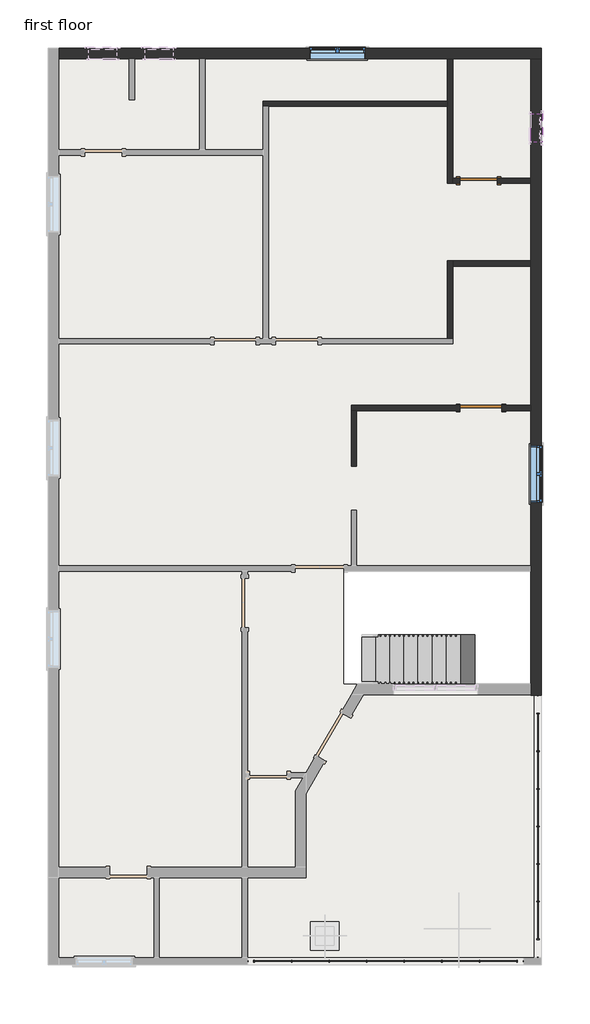
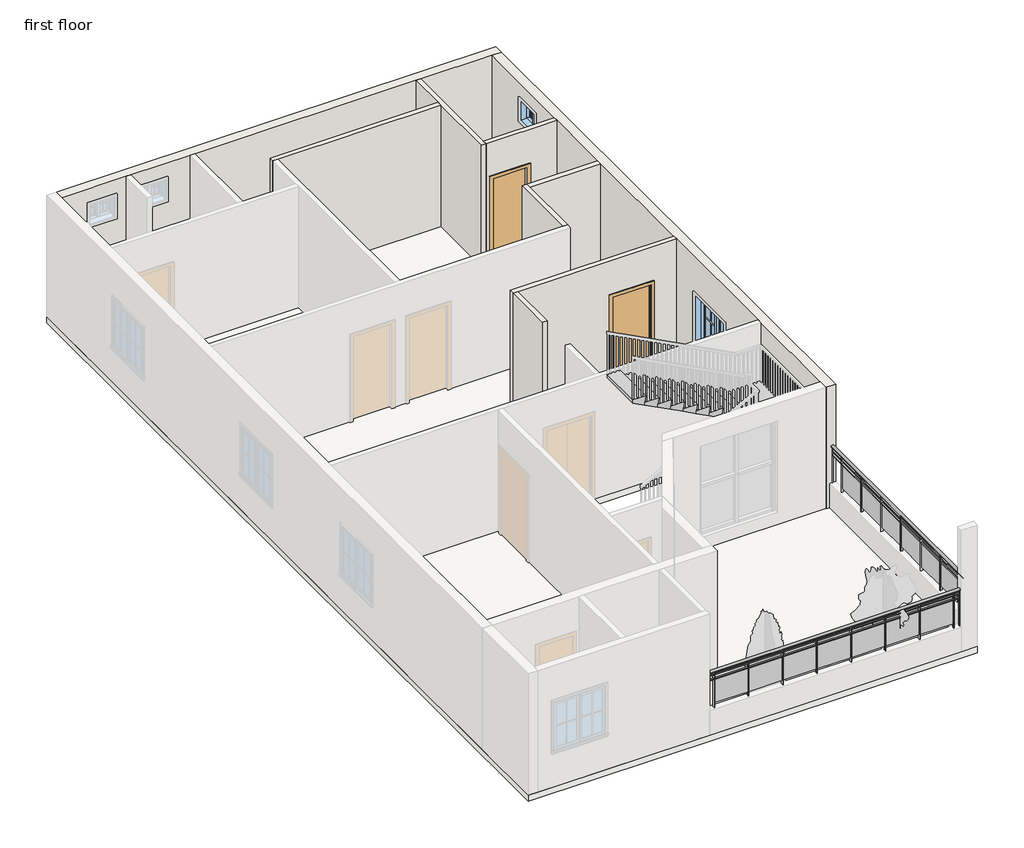
# One storey, part 2 of 4: 9 walls, 3 windows, 2 doors, 2 railings, 1 slab, 1 stair flight.
"""IFC4 building model written with IfcOpenShell, lengths in millimetres."""

from ifc_helpers import new_model, si_unit, point, frame, origin, place, context, project, spatial, polyline, ellipse_curve, trimmed, outline, extrude, faceted_brep, transform, mapped, element, save
from ifc_brep_helpers import plane_surface, extruded_surface, advanced_brep
from components import door_38851409, single_flush_3_x7_305aa2a5, window_79894727, window_casement_double_4_x4_af3140d2

model = new_model("IFC4")

# Units and contexts
model_context = context("Model", 3, world=origin())
ifc_project = project(units=[si_unit("LENGTHUNIT", "METRE", prefix="MILLI")], contexts=[model_context])

# Site, building, storey
site = spatial("IfcSite", under=ifc_project)
building = spatial("IfcBuilding", under=site)
storey = spatial("IfcBuildingStorey", under=building, Name="first floor", Elevation=3200.4)

# Doors
placement = place(None, origin())
door_shape = door_38851409(model_context)
element("IfcDoor", 1, ObjectType="Single-Flush : 2'8\"X7'", at=placement, inside=storey, context=model_context, shape_type="MappedRepresentation", body=[
    mapped(door_shape, transform((3538.5585096, 7293.9976094, 3200.4), x_axis=(-1.0, 0.0, 0.0), y_axis=(0.0, -1.0, 0.0), z_axis=(0.0, 0.0, 1.0))),
])
single_flush_3_x7_shape = single_flush_3_x7_305aa2a5(model_context)
element("IfcDoor", 2, ObjectType="Single-Flush : 3'X7'", at=placement, inside=storey, context=model_context, shape_type="MappedRepresentation", body=[
    mapped(single_flush_3_x7_shape, transform((3589.3585096, 2379.0976094, 3200.4), x_axis=(-1.0, 0.0, 0.0), y_axis=(0.0, -1.0, 0.0), z_axis=(0.0, 0.0, 1.0))),
])

# Railings
element("IfcRailing", 3, ObjectType="Glass Panel - Bottom Fill", at=placement, inside=storey, context=model_context, shape_type="SolidModel", body=[
    advanced_brep(
    [(-1465.2414904, -9539.8523906, 4724.4), (-1465.2414904, -9616.0523906, 4724.4), (4516.4585096, -9539.8523906, 4724.4), (4516.4585096, -9616.0523906, 4724.4)],
    [
        (0, 1, ellipse_curve(frame((-1465.2414904, -9577.9523906, 4724.4), z_axis=(-1.0, 0.0, 0.0), x_axis=(0.0, -1.0, 0.0)), 38.1, 28.575)),
        (1, 0, ellipse_curve(frame((-1465.2414904, -9577.9523906, 4724.4), z_axis=(-1.0, 0.0, 0.0), x_axis=(0.0, -1.0, 0.0)), 38.1, 28.575)),
        (2, 3, ellipse_curve(frame((4516.4585096, -9577.9523906, 4724.4), z_axis=(1.0, 0.0, 0.0), x_axis=(0.0, -1.0, 0.0)), 38.1, 28.575)),
        (3, 2, ellipse_curve(frame((4516.4585096, -9577.9523906, 4724.4), z_axis=(1.0, 0.0, 0.0), x_axis=(0.0, -1.0, 0.0)), 38.1, 28.575)),
        (0, 2),
        (3, 1),
    ],
    [
        plane_surface(frame((-1465.2414904, -9577.9523906, 4724.4), z_axis=(-1.0, 0.0, 0.0), x_axis=(0.0, 1.0, 0.0))),
        plane_surface(frame((4516.4585096, -9577.9523906, 4724.4), z_axis=(1.0, 0.0, 0.0), x_axis=(0.0, 1.0, 0.0))),
        extruded_surface(trimmed(ellipse_curve(frame((4516.4585096, -9577.9523906, 4724.4), z_axis=(-1.0, 0.0, 0.0), x_axis=(0.0, -1.0, 0.0)), 38.1, 28.575), [point((4516.4585096, -9539.8523906, 4724.4))], [point((4516.4585096, -9616.0523906, 4724.4))], True, "CARTESIAN"), (-5981.7, 0.0, 0.0), 5981.7),
        extruded_surface(trimmed(ellipse_curve(frame((4516.4585096, -9577.9523906, 4724.4), z_axis=(-1.0, 0.0, 0.0), x_axis=(0.0, -1.0, 0.0)), 38.1, 28.575), [point((4516.4585096, -9616.0523906, 4724.4))], [point((4516.4585096, -9539.8523906, 4724.4))], True, "CARTESIAN"), (-5981.7, 0.0, 0.0), 5981.7),
    ],
    [
        (0, [[1, 2]]),
        (1, [[3, 4]]),
        (2, [[-1, 5, -4, 6]]),
        (3, [[-2, -6, -3, -5]]),
    ],
),
    extrude(outline(polyline([(-1465.2414904, -9590.6523906), (-1465.2414904, -9565.2523906), (4516.4585096, -9565.2523906), (4516.4585096, -9590.6523906), (-1465.2414904, -9590.6523906)])), frame((0.0, 0.0, 4610.1), z_axis=(0.0, 0.0, 1.0), x_axis=(1.0, 0.0, 0.0)), (0.0, 0.0, 1.0), 25.4),
    extrude(outline(polyline([(-1465.2414904, -9590.6523906), (-1465.2414904, -9565.2523906), (4516.4585096, -9565.2523906), (4516.4585096, -9590.6523906), (-1465.2414904, -9590.6523906)])), frame((0.0, 0.0, 4508.5), z_axis=(0.0, 0.0, 1.0), x_axis=(1.0, 0.0, 0.0)), (0.0, 0.0, 1.0), 25.4),
    extrude(outline(polyline([(4364.0585096, -9603.3523906), (4364.0585096, -9552.5523906), (4376.7585096, -9552.5523906), (4376.7585096, -9603.3523906), (4364.0585096, -9603.3523906)])), frame((0.0, 0.0, 3810.0), z_axis=(0.0, 0.0, 1.0), x_axis=(1.0, 0.0, 0.0)), (0.0, 0.0, 1.0), 885.825),
    extrude(outline(polyline([(3557.6085096, -9571.4172336), (4370.4085096, -9571.4172336), (4370.4085096, -9577.7672336), (3557.6085096, -9577.7672336), (3557.6085096, -9571.4172336)])), frame((0.0, 0.0, 3911.6), z_axis=(0.0, 0.0, 1.0), x_axis=(1.0, 0.0, 0.0)), (0.0, 0.0, 1.0), 596.9),
    extrude(outline(polyline([(3551.2585096, -9603.3523906), (3551.2585096, -9552.5523906), (3563.9585096, -9552.5523906), (3563.9585096, -9603.3523906), (3551.2585096, -9603.3523906)])), frame((0.0, 0.0, 3810.0), z_axis=(0.0, 0.0, 1.0), x_axis=(1.0, 0.0, 0.0)), (0.0, 0.0, 1.0), 885.825),
    extrude(outline(polyline([(2744.8085096, -9571.4172336), (3557.6085096, -9571.4172336), (3557.6085096, -9577.7672336), (2744.8085096, -9577.7672336), (2744.8085096, -9571.4172336)])), frame((0.0, 0.0, 3911.6), z_axis=(0.0, 0.0, 1.0), x_axis=(1.0, 0.0, 0.0)), (0.0, 0.0, 1.0), 596.9),
    extrude(outline(polyline([(2738.4585096, -9603.3523906), (2738.4585096, -9552.5523906), (2751.1585096, -9552.5523906), (2751.1585096, -9603.3523906), (2738.4585096, -9603.3523906)])), frame((0.0, 0.0, 3810.0), z_axis=(0.0, 0.0, 1.0), x_axis=(1.0, 0.0, 0.0)), (0.0, 0.0, 1.0), 885.825),
    extrude(outline(polyline([(1932.0085096, -9571.4172336), (2744.8085096, -9571.4172336), (2744.8085096, -9577.7672336), (1932.0085096, -9577.7672336), (1932.0085096, -9571.4172336)])), frame((0.0, 0.0, 3911.6), z_axis=(0.0, 0.0, 1.0), x_axis=(1.0, 0.0, 0.0)), (0.0, 0.0, 1.0), 596.9),
    extrude(outline(polyline([(1925.6585096, -9603.3523906), (1925.6585096, -9552.5523906), (1938.3585096, -9552.5523906), (1938.3585096, -9603.3523906), (1925.6585096, -9603.3523906)])), frame((0.0, 0.0, 3810.0), z_axis=(0.0, 0.0, 1.0), x_axis=(1.0, 0.0, 0.0)), (0.0, 0.0, 1.0), 885.825),
    extrude(outline(polyline([(1119.2085096, -9571.4172336), (1932.0085096, -9571.4172336), (1932.0085096, -9577.7672336), (1119.2085096, -9577.7672336), (1119.2085096, -9571.4172336)])), frame((0.0, 0.0, 3911.6), z_axis=(0.0, 0.0, 1.0), x_axis=(1.0, 0.0, 0.0)), (0.0, 0.0, 1.0), 596.9),
    extrude(outline(polyline([(1112.8585096, -9603.3523906), (1112.8585096, -9552.5523906), (1125.5585096, -9552.5523906), (1125.5585096, -9603.3523906), (1112.8585096, -9603.3523906)])), frame((0.0, 0.0, 3810.0), z_axis=(0.0, 0.0, 1.0), x_axis=(1.0, 0.0, 0.0)), (0.0, 0.0, 1.0), 885.825),
    extrude(outline(polyline([(306.4085096, -9571.4172336), (1119.2085096, -9571.4172336), (1119.2085096, -9577.7672336), (306.4085096, -9577.7672336), (306.4085096, -9571.4172336)])), frame((0.0, 0.0, 3911.6), z_axis=(0.0, 0.0, 1.0), x_axis=(1.0, 0.0, 0.0)), (0.0, 0.0, 1.0), 596.9),
    extrude(outline(polyline([(300.0585096, -9603.3523906), (300.0585096, -9552.5523906), (312.7585096, -9552.5523906), (312.7585096, -9603.3523906), (300.0585096, -9603.3523906)])), frame((0.0, 0.0, 3810.0), z_axis=(0.0, 0.0, 1.0), x_axis=(1.0, 0.0, 0.0)), (0.0, 0.0, 1.0), 885.825),
    extrude(outline(polyline([(-506.3914904, -9571.4172336), (306.4085096, -9571.4172336), (306.4085096, -9577.7672336), (-506.3914904, -9577.7672336), (-506.3914904, -9571.4172336)])), frame((0.0, 0.0, 3911.6), z_axis=(0.0, 0.0, 1.0), x_axis=(1.0, 0.0, 0.0)), (0.0, 0.0, 1.0), 596.9),
    extrude(outline(polyline([(-512.7414904, -9603.3523906), (-512.7414904, -9552.5523906), (-500.0414904, -9552.5523906), (-500.0414904, -9603.3523906), (-512.7414904, -9603.3523906)])), frame((0.0, 0.0, 3810.0), z_axis=(0.0, 0.0, 1.0), x_axis=(1.0, 0.0, 0.0)), (0.0, 0.0, 1.0), 885.825),
    extrude(outline(polyline([(-1319.1914904, -9571.4172336), (-506.3914904, -9571.4172336), (-506.3914904, -9577.7672336), (-1319.1914904, -9577.7672336), (-1319.1914904, -9571.4172336)])), frame((0.0, 0.0, 3911.6), z_axis=(0.0, 0.0, 1.0), x_axis=(1.0, 0.0, 0.0)), (0.0, 0.0, 1.0), 596.9),
    extrude(outline(polyline([(-1325.5414904, -9603.3523906), (-1325.5414904, -9552.5523906), (-1312.8414904, -9552.5523906), (-1312.8414904, -9603.3523906), (-1325.5414904, -9603.3523906)])), frame((0.0, 0.0, 3810.0), z_axis=(0.0, 0.0, 1.0), x_axis=(1.0, 0.0, 0.0)), (0.0, 0.0, 1.0), 885.825),
    extrude(outline(polyline([(4503.7585096, -9587.4773906), (4503.7585096, -9568.4273906), (4522.8085096, -9568.4273906), (4522.8085096, -9587.4773906), (4503.7585096, -9587.4773906)])), frame((0.0, 0.0, 3810.0), z_axis=(0.0, 0.0, 1.0), x_axis=(1.0, 0.0, 0.0)), (0.0, 0.0, 1.0), 885.825),
    extrude(outline(polyline([(-1471.5914904, -9587.4773906), (-1471.5914904, -9568.4273906), (-1452.5414904, -9568.4273906), (-1452.5414904, -9587.4773906), (-1471.5914904, -9587.4773906)])), frame((0.0, 0.0, 3810.0), z_axis=(0.0, 0.0, 1.0), x_axis=(1.0, 0.0, 0.0)), (0.0, 0.0, 1.0), 885.825),
])
element("IfcRailing", 4, ObjectType="Glass Panel - Bottom Fill", at=placement, inside=storey, context=model_context, shape_type="SolidModel", body=[
    advanced_brep(
    [(4859.3585096, -3824.8523906, 4724.4), (4783.1585096, -3824.8523906, 4724.4), (4859.3585096, -9501.7523906, 4724.4), (4783.1585096, -9501.7523906, 4724.4)],
    [
        (0, 1, ellipse_curve(frame((4821.2585096, -3824.8523906, 4724.4), z_axis=(0.0, 1.0, 0.0), x_axis=(-1.0, 0.0, 0.0)), 38.1, 28.575)),
        (1, 0, ellipse_curve(frame((4821.2585096, -3824.8523906, 4724.4), z_axis=(0.0, 1.0, 0.0), x_axis=(-1.0, 0.0, 0.0)), 38.1, 28.575)),
        (2, 3, ellipse_curve(frame((4821.2585096, -9501.7523906, 4724.4), z_axis=(0.0, -1.0, 0.0), x_axis=(-1.0, 0.0, 0.0)), 38.1, 28.575)),
        (3, 2, ellipse_curve(frame((4821.2585096, -9501.7523906, 4724.4), z_axis=(0.0, -1.0, 0.0), x_axis=(-1.0, 0.0, 0.0)), 38.1, 28.575)),
        (0, 2),
        (3, 1),
    ],
    [
        plane_surface(frame((4821.2585096, -3824.8523906, 4724.4), z_axis=(0.0, 1.0, 0.0), x_axis=(0.0, 0.0, -1.0))),
        plane_surface(frame((4821.2585096, -9501.7523906, 4724.4), z_axis=(0.0, -1.0, 0.0), x_axis=(0.0, 0.0, -1.0))),
        extruded_surface(trimmed(ellipse_curve(frame((4821.2585096, -9501.7523906, 4724.4), z_axis=(0.0, 1.0, 0.0), x_axis=(-1.0, 0.0, 0.0)), 38.1, 28.575), [point((4859.3585096, -9501.7523906, 4724.4))], [point((4783.1585096, -9501.7523906, 4724.4))], True, "CARTESIAN"), (0.0, 5676.900000000001, 0.0), 5676.900000000001),
        extruded_surface(trimmed(ellipse_curve(frame((4821.2585096, -9501.7523906, 4724.4), z_axis=(0.0, 1.0, 0.0), x_axis=(-1.0, 0.0, 0.0)), 38.1, 28.575), [point((4783.1585096, -9501.7523906, 4724.4))], [point((4859.3585096, -9501.7523906, 4724.4))], True, "CARTESIAN"), (0.0, 5676.900000000001, 0.0), 5676.900000000001),
    ],
    [
        (0, [[1, 2]]),
        (1, [[3, 4]]),
        (2, [[-1, 5, -4, 6]]),
        (3, [[-2, -6, -3, -5]]),
    ],
),
    extrude(outline(polyline([(4808.5585096, -3824.8523906), (4833.9585096, -3824.8523906), (4833.9585096, -9501.7523906), (4808.5585096, -9501.7523906), (4808.5585096, -3824.8523906)])), frame((0.0, 0.0, 4610.1), z_axis=(0.0, 0.0, 1.0), x_axis=(1.0, 0.0, 0.0)), (0.0, 0.0, 1.0), 25.4),
    extrude(outline(polyline([(4808.5585096, -3824.8523906), (4833.9585096, -3824.8523906), (4833.9585096, -9501.7523906), (4808.5585096, -9501.7523906), (4808.5585096, -3824.8523906)])), frame((0.0, 0.0, 4508.5), z_axis=(0.0, 0.0, 1.0), x_axis=(1.0, 0.0, 0.0)), (0.0, 0.0, 1.0), 25.4),
    extrude(outline(polyline([(4795.8585096, -9095.3523906), (4846.6585096, -9095.3523906), (4846.6585096, -9108.0523906), (4795.8585096, -9108.0523906), (4795.8585096, -9095.3523906)])), frame((0.0, 0.0, 3810.0), z_axis=(0.0, 0.0, 1.0), x_axis=(1.0, 0.0, 0.0)), (0.0, 0.0, 1.0), 885.825),
    extrude(outline(polyline([(4827.7936666, -8288.9023906), (4827.7936666, -9101.7023906), (4821.4436666, -9101.7023906), (4821.4436666, -8288.9023906), (4827.7936666, -8288.9023906)])), frame((0.0, 0.0, 3911.6), z_axis=(0.0, 0.0, 1.0), x_axis=(1.0, 0.0, 0.0)), (0.0, 0.0, 1.0), 596.9),
    extrude(outline(polyline([(4795.8585096, -8282.5523906), (4846.6585096, -8282.5523906), (4846.6585096, -8295.2523906), (4795.8585096, -8295.2523906), (4795.8585096, -8282.5523906)])), frame((0.0, 0.0, 3810.0), z_axis=(0.0, 0.0, 1.0), x_axis=(1.0, 0.0, 0.0)), (0.0, 0.0, 1.0), 885.825),
    extrude(outline(polyline([(4827.7936666, -7476.1023906), (4827.7936666, -8288.9023906), (4821.4436666, -8288.9023906), (4821.4436666, -7476.1023906), (4827.7936666, -7476.1023906)])), frame((0.0, 0.0, 3911.6), z_axis=(0.0, 0.0, 1.0), x_axis=(1.0, 0.0, 0.0)), (0.0, 0.0, 1.0), 596.9),
    extrude(outline(polyline([(4795.8585096, -7469.7523906), (4846.6585096, -7469.7523906), (4846.6585096, -7482.4523906), (4795.8585096, -7482.4523906), (4795.8585096, -7469.7523906)])), frame((0.0, 0.0, 3810.0), z_axis=(0.0, 0.0, 1.0), x_axis=(1.0, 0.0, 0.0)), (0.0, 0.0, 1.0), 885.825),
    extrude(outline(polyline([(4827.7936666, -6663.3023906), (4827.7936666, -7476.1023906), (4821.4436666, -7476.1023906), (4821.4436666, -6663.3023906), (4827.7936666, -6663.3023906)])), frame((0.0, 0.0, 3911.6), z_axis=(0.0, 0.0, 1.0), x_axis=(1.0, 0.0, 0.0)), (0.0, 0.0, 1.0), 596.9),
    extrude(outline(polyline([(4795.8585096, -6656.9523906), (4846.6585096, -6656.9523906), (4846.6585096, -6669.6523906), (4795.8585096, -6669.6523906), (4795.8585096, -6656.9523906)])), frame((0.0, 0.0, 3810.0), z_axis=(0.0, 0.0, 1.0), x_axis=(1.0, 0.0, 0.0)), (0.0, 0.0, 1.0), 885.825),
    extrude(outline(polyline([(4827.7936666, -5850.5023906), (4827.7936666, -6663.3023906), (4821.4436666, -6663.3023906), (4821.4436666, -5850.5023906), (4827.7936666, -5850.5023906)])), frame((0.0, 0.0, 3911.6), z_axis=(0.0, 0.0, 1.0), x_axis=(1.0, 0.0, 0.0)), (0.0, 0.0, 1.0), 596.9),
    extrude(outline(polyline([(4795.8585096, -5844.1523906), (4846.6585096, -5844.1523906), (4846.6585096, -5856.8523906), (4795.8585096, -5856.8523906), (4795.8585096, -5844.1523906)])), frame((0.0, 0.0, 3810.0), z_axis=(0.0, 0.0, 1.0), x_axis=(1.0, 0.0, 0.0)), (0.0, 0.0, 1.0), 885.825),
    extrude(outline(polyline([(4827.7936666, -5037.7023906), (4827.7936666, -5850.5023906), (4821.4436666, -5850.5023906), (4821.4436666, -5037.7023906), (4827.7936666, -5037.7023906)])), frame((0.0, 0.0, 3911.6), z_axis=(0.0, 0.0, 1.0), x_axis=(1.0, 0.0, 0.0)), (0.0, 0.0, 1.0), 596.9),
    extrude(outline(polyline([(4795.8585096, -5031.3523906), (4846.6585096, -5031.3523906), (4846.6585096, -5044.0523906), (4795.8585096, -5044.0523906), (4795.8585096, -5031.3523906)])), frame((0.0, 0.0, 3810.0), z_axis=(0.0, 0.0, 1.0), x_axis=(1.0, 0.0, 0.0)), (0.0, 0.0, 1.0), 885.825),
    extrude(outline(polyline([(4827.7936666, -4224.9023906), (4827.7936666, -5037.7023906), (4821.4436666, -5037.7023906), (4821.4436666, -4224.9023906), (4827.7936666, -4224.9023906)])), frame((0.0, 0.0, 3911.6), z_axis=(0.0, 0.0, 1.0), x_axis=(1.0, 0.0, 0.0)), (0.0, 0.0, 1.0), 596.9),
    extrude(outline(polyline([(4795.8585096, -4218.5523906), (4846.6585096, -4218.5523906), (4846.6585096, -4231.2523906), (4795.8585096, -4231.2523906), (4795.8585096, -4218.5523906)])), frame((0.0, 0.0, 3810.0), z_axis=(0.0, 0.0, 1.0), x_axis=(1.0, 0.0, 0.0)), (0.0, 0.0, 1.0), 885.825),
    extrude(outline(polyline([(4811.7335096, -9489.0523906), (4830.7835096, -9489.0523906), (4830.7835096, -9508.1023906), (4811.7335096, -9508.1023906), (4811.7335096, -9489.0523906)])), frame((0.0, 0.0, 3810.0), z_axis=(0.0, 0.0, 1.0), x_axis=(1.0, 0.0, 0.0)), (0.0, 0.0, 1.0), 885.825),
    extrude(outline(polyline([(4811.7335096, -3818.5023906), (4830.7835096, -3818.5023906), (4830.7835096, -3837.5523906), (4811.7335096, -3837.5523906), (4811.7335096, -3818.5023906)])), frame((0.0, 0.0, 3810.0), z_axis=(0.0, 0.0, 1.0), x_axis=(1.0, 0.0, 0.0)), (0.0, 0.0, 1.0), 885.825),
])

# Slab
element("IfcSlab", 5, ObjectType="6\"", at=placement, inside=storey, context=model_context, shape_type="SweptSolid", body=[
    extrude(outline(polyline([(4897.4585096, 10157.8476094), (4897.4585096, -9654.1523906), (-5772.1289904, -9654.1523906), (-5772.1289904, 10157.8476094), (4897.4585096, 10157.8476094)]), holes=[polyline([(4668.8585096, -1145.1523906), (630.2585096, -1145.1523906), (630.2585096, -3583.5523906), (4668.8585096, -3583.5523906), (4668.8585096, -1145.1523906)])]), frame((0.0, 0.0, 3048.0), z_axis=(0.0, 0.0, 1.0), x_axis=(1.0, 0.0, 0.0)), (0.0, 0.0, 1.0), 152.4),
])

# Stair flight
element("IfcStairFlight", 6, ObjectType="3/4\" Nosing", at=placement, inside=storey, context=model_context, shape_type="Brep", body=[
    faceted_brep([(1011.2585096, -2516.7523906, 3360.42), (1011.2585096, -3583.5523906, 3360.42), (1335.1085096, -3583.5523906, 3360.42), (1335.1085096, -2516.7523906, 3360.42), (1335.1085096, -2516.7523906, 3288.7008331), (1166.9164466, -2516.7523906, 3200.4), (1030.3085096, -2516.7523906, 3200.4), (1030.3085096, -3583.5523906, 3200.4), (1166.9164466, -3583.5523906, 3200.4), (1335.1085096, -3583.5523906, 3288.7008331), (1316.0585096, -2516.7523906, 3520.44), (1316.0585096, -3583.5523906, 3520.44), (1639.9085096, -3583.5523906, 3520.44), (1639.9085096, -2516.7523906, 3520.44), (1639.9085096, -2516.7523906, 3448.7208331), (1639.9085096, -3583.5523906, 3448.7208331), (1620.8585096, -2516.7523906, 3680.46), (1620.8585096, -3583.5523906, 3680.46), (1944.7085096, -3583.5523906, 3680.46), (1944.7085096, -2516.7523906, 3680.46), (1944.7085096, -2516.7523906, 3608.7408331), (1944.7085096, -3583.5523906, 3608.7408331), (1925.6585096, -2516.7523906, 3840.48), (1925.6585096, -3583.5523906, 3840.48), (2249.5085096, -3583.5523906, 3840.48), (2249.5085096, -2516.7523906, 3840.48), (2249.5085096, -2516.7523906, 3768.7608331), (2249.5085096, -3583.5523906, 3768.7608331), (2230.4585096, -2516.7523906, 4000.5), (2230.4585096, -3583.5523906, 4000.5), (2554.3085096, -3583.5523906, 4000.5), (2554.3085096, -2516.7523906, 4000.5), (2554.3085096, -2516.7523906, 3928.7808331), (2554.3085096, -3583.5523906, 3928.7808331), (2535.2585096, -2516.7523906, 4160.52), (2535.2585096, -3583.5523906, 4160.52), (2859.1085096, -3583.5523906, 4160.52), (2859.1085096, -2516.7523906, 4160.52), (2859.1085096, -2516.7523906, 4088.8008331), (2859.1085096, -3583.5523906, 4088.8008331), (2840.0585096, -2516.7523906, 4320.54), (2840.0585096, -3583.5523906, 4320.54), (3163.9085096, -3583.5523906, 4320.54), (3163.9085096, -2516.7523906, 4320.54), (3163.9085096, -2516.7523906, 4248.8208331), (3163.9085096, -3583.5523906, 4248.8208331), (3144.8585096, -2516.7523906, 4480.56), (3144.8585096, -3583.5523906, 4480.56), (3468.7085096, -3583.5523906, 4480.56), (3468.7085096, -2516.7523906, 4480.56), (3468.7085096, -2516.7523906, 4408.8408331), (3468.7085096, -3583.5523906, 4408.8408331), (3773.5085096, -2516.7523906, 4640.58), (3449.6585096, -2516.7523906, 4640.58), (3449.6585096, -3583.5523906, 4640.58), (3773.5085096, -3583.5523906, 4640.58), (3762.0180334, -2516.7523906, 4737.1), (4093.9640656, -2516.7523906, 4737.1), (3773.5085096, -3583.5523906, 4568.8608331), (3735.4085096, -2211.9523906, 4800.6), (3754.4585096, -2211.9523906, 4800.6), (3754.4585096, -2516.7523906, 4800.6), (3754.4585096, -3583.5523906, 4800.6), (4093.9640656, -3583.5523906, 4800.6), (4668.8585096, -3583.5523906, 4800.6), (4668.8585096, -1145.1523906, 4800.6), (3735.4085096, -1145.1523906, 4800.6), (3735.4085096, -2211.9523906, 4737.1), (3754.4585096, -2211.9523906, 4737.1), (3754.4585096, -2516.7523906, 4737.1), (4093.9640656, -3583.5523906, 4737.1), (4668.8585096, -3583.5523906, 4737.1), (4668.8585096, -1145.1523906, 4737.1), (3735.4085096, -1145.1523906, 4737.1), (3754.4585096, -2211.9523906, 4960.62), (3754.4585096, -1145.1523906, 4960.62), (3719.7529535, -1145.1523906, 4960.62), (3430.6085096, -1145.1523906, 4960.62), (3430.6085096, -2211.9523906, 4960.62), (3719.7529535, -2211.9523906, 4960.62), (3430.6085096, -2211.9523906, 4888.9008331), (3719.7529535, -2211.9523906, 4737.1), (3719.7529535, -1145.1523906, 4737.1), (3430.6085096, -1145.1523906, 4888.9008331), (3449.6585096, -2211.9523906, 5120.64), (3449.6585096, -1145.1523906, 5120.64), (3125.8085096, -1145.1523906, 5120.64), (3125.8085096, -2211.9523906, 5120.64), (3125.8085096, -2211.9523906, 5048.9208331), (3125.8085096, -1145.1523906, 5048.9208331), (3144.8585096, -2211.9523906, 5280.66), (3144.8585096, -1145.1523906, 5280.66), (2821.0085096, -1145.1523906, 5280.66), (2821.0085096, -2211.9523906, 5280.66), (2821.0085096, -2211.9523906, 5208.9408331), (2821.0085096, -1145.1523906, 5208.9408331), (2840.0585096, -2211.9523906, 5440.68), (2840.0585096, -1145.1523906, 5440.68), (2516.2085096, -1145.1523906, 5440.68), (2516.2085096, -2211.9523906, 5440.68), (2516.2085096, -2211.9523906, 5368.9608331), (2516.2085096, -1145.1523906, 5368.9608331), (2535.2585096, -2211.9523906, 5600.7), (2535.2585096, -1145.1523906, 5600.7), (2211.4085096, -1145.1523906, 5600.7), (2211.4085096, -2211.9523906, 5600.7), (2211.4085096, -2211.9523906, 5528.9808331), (2211.4085096, -1145.1523906, 5528.9808331), (2230.4585096, -2211.9523906, 5760.72), (2230.4585096, -1145.1523906, 5760.72), (1906.6085096, -1145.1523906, 5760.72), (1906.6085096, -2211.9523906, 5760.72), (1906.6085096, -2211.9523906, 5689.0008331), (1906.6085096, -1145.1523906, 5689.0008331), (1925.6585096, -2211.9523906, 5920.74), (1925.6585096, -1145.1523906, 5920.74), (1601.8085096, -1145.1523906, 5920.74), (1601.8085096, -2211.9523906, 5920.74), (1601.8085096, -2211.9523906, 5849.0208331), (1601.8085096, -1145.1523906, 5849.0208331), (1620.8585096, -2211.9523906, 6080.76), (1620.8585096, -1145.1523906, 6080.76), (1297.0085096, -1145.1523906, 6080.76), (1297.0085096, -2211.9523906, 6080.76), (1297.0085096, -2211.9523906, 6009.0408331), (1297.0085096, -1145.1523906, 6009.0408331), (1316.0585096, -2211.9523906, 6240.78), (1316.0585096, -1145.1523906, 6240.78), (1011.2585096, -1145.1523906, 6240.78), (1011.2585096, -2211.9523906, 6240.78), (1011.2585096, -2211.9523906, 6159.0595831), (1011.2585096, -1145.1523906, 6159.0595831)], [[[0, 1, 2, 3]], [[0, 3, 4, 5, 6]], [[2, 1, 7, 8, 9]], [[10, 11, 12, 13]], [[10, 13, 14, 4, 3]], [[12, 11, 2, 9, 15]], [[16, 17, 18, 19]], [[16, 19, 20, 14, 13]], [[18, 17, 12, 15, 21]], [[22, 23, 24, 25]], [[22, 25, 26, 20, 19]], [[24, 23, 18, 21, 27]], [[28, 29, 30, 31]], [[28, 31, 32, 26, 25]], [[30, 29, 24, 27, 33]], [[34, 35, 36, 37]], [[34, 37, 38, 32, 31]], [[36, 35, 30, 33, 39]], [[40, 41, 42, 43]], [[40, 43, 44, 38, 37]], [[42, 41, 36, 39, 45]], [[46, 47, 48, 49]], [[46, 49, 50, 44, 43]], [[48, 47, 42, 45, 51]], [[52, 53, 54, 55]], [[52, 56, 57, 50, 49, 53]], [[55, 54, 48, 51, 58]], [[59, 60, 61, 62, 63, 64, 65, 66]], [[60, 59, 67, 68]], [[61, 60, 68, 69]], [[56, 61, 69]], [[62, 55, 58, 70, 71, 64, 63]], [[65, 64, 71, 72]], [[66, 65, 72, 73]], [[74, 75, 76, 77, 78, 79]], [[59, 74, 79, 78, 80, 81, 67]], [[75, 66, 73, 82, 83, 77, 76]], [[84, 85, 86, 87]], [[84, 87, 88, 80, 78]], [[86, 85, 77, 83, 89]], [[90, 91, 92, 93]], [[90, 93, 94, 88, 87]], [[92, 91, 86, 89, 95]], [[96, 97, 98, 99]], [[96, 99, 100, 94, 93]], [[98, 97, 92, 95, 101]], [[102, 103, 104, 105]], [[102, 105, 106, 100, 99]], [[104, 103, 98, 101, 107]], [[108, 109, 110, 111]], [[108, 111, 112, 106, 105]], [[110, 109, 104, 107, 113]], [[114, 115, 116, 117]], [[114, 117, 118, 112, 111]], [[116, 115, 110, 113, 119]], [[120, 121, 122, 123]], [[120, 123, 124, 118, 117]], [[122, 121, 116, 119, 125]], [[1, 0, 6, 7]], [[3, 2, 11, 10]], [[13, 12, 17, 16]], [[19, 18, 23, 22]], [[25, 24, 29, 28]], [[31, 30, 35, 34]], [[37, 36, 41, 40]], [[43, 42, 47, 46]], [[49, 48, 54, 53]], [[52, 55, 62, 61, 56]], [[59, 66, 75, 74]], [[78, 77, 85, 84]], [[87, 86, 91, 90]], [[93, 92, 97, 96]], [[99, 98, 103, 102]], [[105, 104, 109, 108]], [[111, 110, 115, 114]], [[117, 116, 121, 120]], [[126, 127, 128, 129]], [[126, 129, 130, 124, 123]], [[128, 127, 122, 125, 131]], [[129, 128, 131, 130]], [[123, 122, 127, 126]], [[7, 6, 5, 8]], [[50, 57, 70, 58, 51, 45, 39, 33, 27, 21, 15, 9, 8, 5, 4, 14, 20, 26, 32, 38, 44]], [[70, 57, 56, 69, 68, 67, 81, 82, 73, 72, 71]], [[82, 81, 80, 88, 94, 100, 106, 112, 118, 124, 130, 131, 125, 119, 113, 107, 101, 95, 89, 83]]]),
])

# Walls
element("IfcWall", 7, ObjectType="4.5\"", at=placement, inside=storey, context=model_context, shape_type="Brep", body=[
    faceted_brep([(2979.7585096, 3884.0476094, 3200.4), (2979.7585096, 5446.1476094, 3200.4), (2979.7585096, 5560.4476094, 3200.4), (2979.7585096, 5560.4476094, 6248.4), (2979.7585096, 5446.1476094, 6248.4), (2979.7585096, 3884.0476094, 6248.4), (2865.4585096, 3884.0476094, 3200.4), (2865.4585096, 3884.0476094, 6248.4), (2865.4585096, 5560.4476094, 6248.4), (2865.4585096, 5560.4476094, 3200.4)], [[[0, 1, 2, 3, 4, 5]], [[6, 7, 8, 9]], [[2, 1, 0, 6, 9]], [[5, 4, 3, 8, 7]], [[0, 5, 7, 6]], [[3, 2, 9, 8]]]),
])
element("IfcWall", 8, ObjectType="4.5\"", at=placement, inside=storey, context=model_context, shape_type="SweptSolid", body=[
    extrude(outline(polyline([(4668.8585096, 5446.1476094), (2979.7585096, 5446.1476094), (2979.7585096, 5560.4476094), (4668.8585096, 5560.4476094), (4668.8585096, 5446.1476094)])), frame((0.0, 0.0, 3200.4), z_axis=(0.0, 0.0, 1.0), x_axis=(1.0, 0.0, 0.0)), (0.0, 0.0, 1.0), 3048.0),
])
element("IfcWall", 9, ObjectType="4.5\"", at=placement, inside=storey, context=model_context, shape_type="Brep", body=[
    faceted_brep([(3132.1585096, 2436.2476094, 5334.0), (3132.1585096, 2436.2476094, 3200.4), (782.6585096, 2436.2476094, 3200.4), (782.6585096, 2436.2476094, 6248.4), (4668.8585096, 2436.2476094, 6248.4), (4668.8585096, 2436.2476094, 3200.4), (4046.5585096, 2436.2476094, 3200.4), (4046.5585096, 2436.2476094, 5334.0), (782.6585096, 2321.9476094, 3200.4), (896.9585096, 2321.9476094, 3200.4), (3132.1585096, 2321.9476094, 3200.4), (3132.1585096, 2321.9476094, 5334.0), (4046.5585096, 2321.9476094, 5334.0), (4046.5585096, 2321.9476094, 3200.4), (4668.8585096, 2321.9476094, 3200.4), (4668.8585096, 2321.9476094, 6248.4), (896.9585096, 2321.9476094, 6248.4), (782.6585096, 2321.9476094, 6248.4)], [[[0, 1, 2, 3, 4, 5, 6, 7]], [[8, 9, 10, 11, 12, 13, 14, 15, 16, 17]], [[6, 5, 14, 13]], [[2, 1, 10, 9, 8]], [[4, 3, 17, 16, 15]], [[5, 4, 15, 14]], [[3, 2, 8, 17]], [[11, 10, 1, 0]], [[12, 11, 0, 7]], [[13, 12, 7, 6]]]),
])
element("IfcWall", 10, ObjectType="4.5\"", at=placement, inside=storey, context=model_context, shape_type="SweptSolid", body=[
    extrude(outline(polyline([(782.6585096, 1121.7976094), (782.6585096, 2321.9476094), (896.9585096, 2321.9476094), (896.9585096, 1121.7976094), (782.6585096, 1121.7976094)])), frame((0.0, 0.0, 3200.4), z_axis=(0.0, 0.0, 1.0), x_axis=(1.0, 0.0, 0.0)), (0.0, 0.0, 1.0), 3048.0),
])
element("IfcWall", 11, ObjectType="4.5\"", at=placement, inside=storey, context=model_context, shape_type="Brep", body=[
    faceted_brep([(2865.4585096, 9929.2476094, 3200.4), (2865.4585096, 9014.8476094, 3200.4), (2865.4585096, 8900.5476094, 3200.4), (2865.4585096, 7236.8476094, 3200.4), (2865.4585096, 7236.8476094, 6248.4), (2865.4585096, 8900.5476094, 6248.4), (2865.4585096, 9014.8476094, 6248.4), (2865.4585096, 9929.2476094, 6248.4), (2979.7585096, 9929.2476094, 3200.4), (2979.7585096, 9929.2476094, 6248.4), (2979.7585096, 7351.1476094, 6248.4), (2979.7585096, 7236.8476094, 6248.4), (2979.7585096, 7236.8476094, 3200.4), (2979.7585096, 7351.1476094, 3200.4)], [[[0, 1, 2, 3, 4, 5, 6, 7]], [[8, 9, 10, 11, 12, 13]], [[3, 2, 1, 0, 8, 13, 12]], [[7, 6, 5, 4, 11, 10, 9]], [[0, 7, 9, 8]], [[4, 3, 12, 11]]]),
])
element("IfcWall", 12, ObjectType="4.5\"", at=placement, inside=storey, context=model_context, shape_type="SweptSolid", body=[
    extrude(outline(polyline([(3200.4, 2979.7585096), (3200.4, 3132.1585096), (5334.0, 3132.1585096), (5334.0, 3944.9585096), (3200.4, 3944.9585096), (3200.4, 4668.8585096), (6248.4, 4668.8585096), (6248.4, 2979.7585096), (3200.4, 2979.7585096)])), frame((0.0, 7236.8476094, 0.0), z_axis=(0.0, 1.0, 0.0), x_axis=(0.0, 0.0, 1.0)), (0.0, 0.0, 1.0), 114.3),
])
element("IfcWall", 13, ObjectType="4.5\"", at=placement, inside=storey, context=model_context, shape_type="Brep", body=[
    faceted_brep([(2865.4585096, 9014.8476094, 3200.4), (-1122.3414904, 9014.8476094, 3200.4), (-1122.3414904, 9014.8476094, 6248.4), (2865.4585096, 9014.8476094, 6248.4), (2865.4585096, 8900.5476094, 3200.4), (2865.4585096, 8900.5476094, 6248.4), (-1008.0414904, 8900.5476094, 6248.4), (-1122.3414904, 8900.5476094, 6248.4), (-1122.3414904, 8900.5476094, 3200.4), (-1008.0414904, 8900.5476094, 3200.4)], [[[0, 1, 2, 3]], [[4, 5, 6, 7, 8, 9]], [[1, 0, 4, 9, 8]], [[3, 2, 7, 6, 5]], [[0, 3, 5, 4]], [[2, 1, 8, 7]]]),
])
element("IfcWall", 14, ObjectType="9\" 2", at=placement, inside=storey, context=model_context, shape_type="Brep", body=[
    faceted_brep([(-5543.5289904, 9929.2476094, 3200.4), (-4017.9414904, 9929.2476094, 3200.4), (-3903.6414904, 9929.2476094, 3200.4), (-2493.9414904, 9929.2476094, 3200.4), (-2379.6414904, 9929.2476094, 3200.4), (2865.4585096, 9929.2476094, 3200.4), (2979.7585096, 9929.2476094, 3200.4), (4668.8585096, 9929.2476094, 3200.4), (4897.4585096, 9929.2476094, 3200.4), (4897.4585096, 9929.2476094, 6248.4), (4668.8585096, 9929.2476094, 6248.4), (2979.7585096, 9929.2476094, 6248.4), (2865.4585096, 9929.2476094, 6248.4), (-2379.6414904, 9929.2476094, 6248.4), (-2493.9414904, 9929.2476094, 6248.4), (-3903.6414904, 9929.2476094, 6248.4), (-4017.9414904, 9929.2476094, 6248.4), (-5543.5289904, 9929.2476094, 6248.4), (-4290.9914904, 9929.2476094, 5867.4), (-4290.9914904, 9929.2476094, 5334.0), (-4900.5914904, 9929.2476094, 5334.0), (-4900.5914904, 9929.2476094, 5867.4), (-3071.7914904, 9929.2476094, 5867.4), (-3071.7914904, 9929.2476094, 5334.0), (-3681.3914904, 9929.2476094, 5334.0), (-3681.3914904, 9929.2476094, 5867.4), (1093.8085096, 9929.2476094, 5334.0), (1093.8085096, 9929.2476094, 4114.8), (-125.3914904, 9929.2476094, 4114.8), (-125.3914904, 9929.2476094, 5334.0), (-5543.5289904, 10157.8476094, 3200.4), (-5543.5289904, 10157.8476094, 6248.4), (4897.4585096, 10157.8476094, 6248.4), (4897.4585096, 10157.8476094, 3200.4), (-4290.9914904, 10157.8476094, 5867.4), (-4900.5914904, 10157.8476094, 5867.4), (-4900.5914904, 10157.8476094, 5334.0), (-4290.9914904, 10157.8476094, 5334.0), (-3071.7914904, 10157.8476094, 5867.4), (-3681.3914904, 10157.8476094, 5867.4), (-3681.3914904, 10157.8476094, 5334.0), (-3071.7914904, 10157.8476094, 5334.0), (1093.8085096, 10157.8476094, 5334.0), (-125.3914904, 10157.8476094, 5334.0), (-125.3914904, 10157.8476094, 4114.8), (1093.8085096, 10157.8476094, 4114.8)], [[[0, 1, 2, 3, 4, 5, 6, 7, 8, 9, 10, 11, 12, 13, 14, 15, 16, 17], [18, 19, 20, 21], [22, 23, 24, 25], [26, 27, 28, 29]], [[30, 31, 32, 33], [34, 35, 36, 37], [38, 39, 40, 41], [42, 43, 44, 45]], [[8, 7, 6, 5, 4, 3, 2, 1, 0, 30, 33]], [[17, 16, 15, 14, 13, 12, 11, 10, 9, 32, 31]], [[0, 17, 31, 30]], [[9, 8, 33, 32]], [[19, 18, 34, 37]], [[20, 19, 37, 36]], [[21, 20, 36, 35]], [[18, 21, 35, 34]], [[23, 22, 38, 41]], [[24, 23, 41, 40]], [[25, 24, 40, 39]], [[22, 25, 39, 38]], [[27, 26, 42, 45]], [[28, 27, 45, 44]], [[29, 28, 44, 43]], [[26, 29, 43, 42]]]),
])
element("IfcWall", 15, ObjectType="9\" 2", at=placement, inside=storey, context=model_context, shape_type="Brep", body=[
    faceted_brep([(4668.8585096, 9929.2476094, 3200.4), (4668.8585096, 7351.1476094, 3200.4), (4668.8585096, 7236.8476094, 3200.4), (4668.8585096, 5560.4476094, 3200.4), (4668.8585096, 5446.1476094, 3200.4), (4668.8585096, 2436.2476094, 3200.4), (4668.8585096, 2321.9476094, 3200.4), (4668.8585096, -1030.8523906, 3200.4), (4668.8585096, -1145.1523906, 3200.4), (4668.8585096, -3583.5523906, 3200.4), (4668.8585096, -3812.1523906, 3200.4), (4668.8585096, -3824.8523906, 3200.4), (4668.8585096, -3824.8523906, 6248.4), (4668.8585096, -3812.1523906, 6248.4), (4668.8585096, -3583.5523906, 6248.4), (4668.8585096, -1145.1523906, 6248.4), (4668.8585096, -1030.8523906, 6248.4), (4668.8585096, 2321.9476094, 6248.4), (4668.8585096, 2436.2476094, 6248.4), (4668.8585096, 5446.1476094, 6248.4), (4668.8585096, 5560.4476094, 6248.4), (4668.8585096, 7236.8476094, 6248.4), (4668.8585096, 7351.1476094, 6248.4), (4668.8585096, 9929.2476094, 6248.4), (4668.8585096, 347.0976094, 5334.0), (4668.8585096, 347.0976094, 4114.8), (4668.8585096, 1566.2976094, 4114.8), (4668.8585096, 1566.2976094, 5334.0), (4668.8585096, 8132.1976094, 5867.4), (4668.8585096, 8132.1976094, 5334.0), (4668.8585096, 8741.7976094, 5334.0), (4668.8585096, 8741.7976094, 5867.4), (4897.4585096, 9929.2476094, 3200.4), (4897.4585096, 9929.2476094, 6248.4), (4897.4585096, -3824.8523906, 6248.4), (4897.4585096, -3824.8523906, 3810.0), (4897.4585096, -3824.8523906, 3200.4), (4897.4585096, 347.0976094, 5334.0), (4897.4585096, 1566.2976094, 5334.0), (4897.4585096, 1566.2976094, 4114.8), (4897.4585096, 347.0976094, 4114.8), (4897.4585096, 8132.1976094, 5867.4), (4897.4585096, 8741.7976094, 5867.4), (4897.4585096, 8741.7976094, 5334.0), (4897.4585096, 8132.1976094, 5334.0), (4745.0585096, -3824.8523906, 3200.4)], [[[0, 1, 2, 3, 4, 5, 6, 7, 8, 9, 10, 11, 12, 13, 14, 15, 16, 17, 18, 19, 20, 21, 22, 23], [24, 25, 26, 27], [28, 29, 30, 31]], [[32, 33, 34, 35, 36], [37, 38, 39, 40], [41, 42, 43, 44]], [[11, 10, 9, 8, 7, 6, 5, 4, 3, 2, 1, 0, 32, 36, 45]], [[12, 11, 45, 36, 35, 34]], [[23, 22, 21, 20, 19, 18, 17, 16, 15, 14, 13, 12, 34, 33]], [[0, 23, 33, 32]], [[25, 24, 37, 40]], [[26, 25, 40, 39]], [[27, 26, 39, 38]], [[24, 27, 38, 37]], [[29, 28, 41, 44]], [[30, 29, 44, 43]], [[31, 30, 43, 42]], [[28, 31, 42, 41]]]),
])

# Windows
window_shape = window_79894727(model_context)
element("IfcWindow", 16, ObjectType="Window-Casement-Double : 2'X1'9\"", at=placement, inside=storey, context=model_context, shape_type="MappedRepresentation", body=[
    mapped(window_shape, transform((4783.1585096, 8436.9976094, 3200.4), x_axis=(0.0, -1.0, 0.0), y_axis=(1.0, 0.0, 0.0), z_axis=(0.0, 0.0, 1.0))),
])
window_casement_double_4_x4_shape = window_casement_double_4_x4_af3140d2(model_context)
element("IfcWindow", 17, ObjectType="Window-Casement-Double : 4'X4'", at=placement, inside=storey, context=model_context, shape_type="MappedRepresentation", body=[
    mapped(window_casement_double_4_x4_shape, transform((4783.1585096, 956.6976094, 3200.4), x_axis=(0.0, -1.0, 0.0), y_axis=(1.0, 0.0, 0.0), z_axis=(0.0, 0.0, 1.0))),
])
element("IfcWindow", 18, ObjectType="Window-Casement-Double : 4'X4'", at=placement, inside=storey, context=model_context, shape_type="MappedRepresentation", body=[
    mapped(window_casement_double_4_x4_shape, transform((484.2085096, 10043.5476094, 3200.4), x_axis=(1.0, 0.0, 0.0), y_axis=(0.0, 1.0, 0.0), z_axis=(0.0, 0.0, 1.0))),
])

save(model, "model.ifc")

# Revit data of these elements
# Type "Single-Flush : 2'8\"X7'"
#   Type Mark = "9"
#   Construction Type Id = "MDOOR"
#   Assembly Code = "C1020"
#   Analytic Construction = "Metal"
#   Thickness = 0' - 2"
#   Heat Transfer Coefficient (U) = 0.651978 BTU/(h·ft²·°F)
#   Height = 7' - 0"
#   Trim Projection Ext = 0' - 1"
#   Trim Projection Int = 0' - 1"
#   Trim Width = 0' - 3"
#   Width = 2' - 8"
#   Define Thermal Properties by = 1
#   Door Material = Door - Panel
#   Frame Material = Door - Frame
#   Visual Light Transmittance = 0
#   Solar Heat Gain Coefficient = 0
#   Function = (empty or 0)
#   Wall Closure = (empty or 0)
# Type "Single-Flush : 3'X7'"
#   Type Mark = "8"
#   Construction Type Id = "MDOOR"
#   Assembly Code = "C1020"
#   Analytic Construction = "Metal"
#   Thickness = 0' - 2"
#   Heat Transfer Coefficient (U) = 0.651978 BTU/(h·ft²·°F)
#   Height = 7' - 0"
#   Trim Projection Ext = 0' - 1"
#   Trim Projection Int = 0' - 1"
#   Trim Width = 0' - 3"
#   Width = 3' - 0"
#   Define Thermal Properties by = 1
#   Door Material = Door - Panel
#   Frame Material = Door - Frame
#   Visual Light Transmittance = 0
#   Solar Heat Gain Coefficient = 0
#   Function = (empty or 0)
#   Wall Closure = (empty or 0)
# Type "Glass Panel - Bottom Fill"
#   Assembly Code = "C2010400"
#   built-in parameter 1008612 = 0.0416667 (stored number, unit not read)
#   built-in parameter 1008611 = 0.0416667 (stored number, unit not read)
#   built-in parameter 1008609 = 0.333333 (stored number, unit not read)
#   built-in parameter 1008604 = 0.166667 (stored number, unit not read)
#   built-in parameter 1008603 = 0.166667 (stored number, unit not read)
#   Railing Height = 3' - 0"
#   built-in parameter 1008630 = 2
#   built-in parameter 1008610 = 2
#   built-in parameter 1008618 = Baluster - Square : 3/4"
# Type "6\""
#   Assembly Code = "B1010"
#   Function = 0
#   Layers, outside or top first: 0' - 6" no material (function 1)
# Type "4.5\""
#   Assembly Code = "B2010"
#   Layers, outside or top first: 0' - 4 1/2" no material (function 1)
# Type "9\" 2"
#   Assembly Code = "B2010"
#   Layers, outside or top first: 0' - 9" "wall" (function 1)
# Type "Window-Casement-Double : 2'X1'9\""
#   Type Mark = "20"
#   Fire Rating = "0.5h"
#   Assembly Code = "B2020100"
#   Analytic Construction = "Double glazing - domestic"
#   Frame Extension [instance default] = 0' - 0 1/4"
#   Window Inset [instance default] = 0' - 0"
#   Wall Thickness [instance default] = 0' - 6"
#   Interior Wall Closure [instance default] = 0' - 2 1/4"
#   Half Width = 1' - 0"
#   Visual Light Transmittance = 0.81
#   Thermal Resistance (R) = 1.8146 (h·ft²·°F)/BTU
#   Solar Heat Gain Coefficient = 0.76
#   Rough Width = 2' - 0 1/2"
#   Rough Height = 1' - 9 1/2"
#   Height = 1' - 9"
#   Heat Transfer Coefficient (U) = 0.5511 BTU/(h·ft²·°F)
#   Exterior Wall Closure [instance default] = 0' - 1 1/4"
#   Extension Jamb [instance default] = 0' - 2 1/4"
#   Default Sill Height = 7' - 0"
#   Width = 2' - 0"
#   Muntin Visibility = yes
#   Interior Trim Visibility [instance default] = yes
#   Exterior Trim Visibility [instance default] = yes
#   Extension Jamb Visibility [instance default] = yes
#   Interior Trim Material = Wood - Stained
#   Muntin Pattern = Muntin Pattern_2x2 : Muntin Pattern_2x2
#   Interior Trim = Trim-Window-Interior-Flat : Picture Frame
#   Interior Frame Material = Wood - Stained
#   Glass Panel Material = Glass
#   Exterior Trim Material = Clad - White
#   Exterior Trim = Trim-Window-Exterior-Flat : with Sill
#   Exterior Frame Material = Clad - White
#   Wall Closure = (empty or 0)
# Type "Window-Casement-Double : 4'X4'"
#   Type Mark = "19"
#   Fire Rating = "0.5h"
#   Assembly Code = "B2020100"
#   Analytic Construction = "Double glazing - domestic"
#   Frame Extension [instance default] = 0' - 0 1/4"
#   Window Inset [instance default] = 0' - 0"
#   Wall Thickness [instance default] = 0' - 6"
#   Interior Wall Closure [instance default] = 0' - 2 1/4"
#   Half Width = 2' - 0"
#   Visual Light Transmittance = 0.81
#   Thermal Resistance (R) = 1.8146 (h·ft²·°F)/BTU
#   Solar Heat Gain Coefficient = 0.76
#   Rough Width = 4' - 0 1/2"
#   Rough Height = 4' - 0 1/2"
#   Height = 4' - 0"
#   Heat Transfer Coefficient (U) = 0.5511 BTU/(h·ft²·°F)
#   Exterior Wall Closure [instance default] = 0' - 1 1/4"
#   Extension Jamb [instance default] = 0' - 2 1/4"
#   Default Sill Height = 3' - 0"
#   Width = 4' - 0"
#   Muntin Visibility = yes
#   Interior Trim Visibility [instance default] = yes
#   Exterior Trim Visibility [instance default] = yes
#   Extension Jamb Visibility [instance default] = yes
#   Interior Trim Material = Wood - Stained
#   Muntin Pattern = Muntin Pattern_2x2 : Muntin Pattern_2x2
#   Interior Trim = Trim-Window-Interior-Flat : Picture Frame
#   Interior Frame Material = Wood - Stained
#   Glass Panel Material = Glass
#   Exterior Trim Material = Clad - White
#   Exterior Trim = Trim-Window-Exterior-Flat : with Sill
#   Exterior Frame Material = Clad - White
#   Wall Closure = (empty or 0)
# Element 1 (IfcDoor, "Single-Flush : 2'8\"X7'")
#   Phase Created = New Construction
#   Materials on its faces: "Door - Frame", "Door - Panel"
# Element 2 (IfcDoor, "Single-Flush : 3'X7'")
#   Phase Created = New Construction
#   Materials on its faces: "Door - Frame", "Door - Panel"
# Elements 3, 4 (IfcRailing, "Glass Panel - Bottom Fill")
#   built-in parameter 1008621 = 2 (stored number, unit not read)
#   Phase Created = New Construction
#   Materials on its faces: "Glass"
# Element 5 (IfcSlab, "6\"")
#   Height Offset From Level = 0' - 0"
#   Phase Created = New Construction
#   Materials on its faces: "wood 1", "Default Floor"
# Element 6 (IfcStairFlight, "3/4\" Nosing")
#   Phase Created = New Construction
#   Materials on its faces: "Concrete, Cast-in-Place gray"
# Elements 7, 8, 9, 10, 11, 12, 13 (IfcWall, "4.5\"")
#   Top Offset = -0' - 6"
#   Base Offset = 0' - 0"
#   wall height = 10' - 0"
#   Phase Created = New Construction
#   Base Constraint = first floor
#   Top Constraint = second floor
#   Materials on its faces: "Default Wall"
# Element 14 (IfcWall, "9\" 2")
#   Top Offset = -0' - 6"
#   Base Offset = 0' - 0"
#   wall height = 10' - 0"
#   Phase Created = New Construction
#   Base Constraint = first floor
#   Top Constraint = second floor
#   Materials on its faces: "wall", "6\" wall", "wall 1"
# Element 15 (IfcWall, "9\" 2")
#   Top Offset = -0' - 6"
#   Base Offset = 0' - 0"
#   wall height = 10' - 0"
#   Phase Created = New Construction
#   Base Constraint = first floor
#   Top Constraint = second floor
#   Materials on its faces: "wall", "wall 1"
# Element 16 (IfcWindow, "Window-Casement-Double : 2'X1'9\"")
#   Mark = "16"
#   Window Inset = 0' - 0"
#   Interior Wall Closure = 0' - 2 1/4"
#   Frame Extension = 0' - 0 1/4"
#   Exterior Wall Closure = 0' - 1 1/4"
#   Interior Trim Visibility = yes
#   Exterior Trim Visibility = yes
#   Phase Created = New Construction
#   Materials on its faces: "Wood - Stained", "Glass", "Clad - White"
# Element 17 (IfcWindow, "Window-Casement-Double : 4'X4'")
#   Mark = "13"
#   Window Inset = 0' - 0"
#   Interior Wall Closure = 0' - 2 1/4"
#   Frame Extension = 0' - 0 1/4"
#   Exterior Wall Closure = 0' - 1 1/4"
#   Interior Trim Visibility = yes
#   Exterior Trim Visibility = yes
#   Phase Created = New Construction
#   Materials on its faces: "Wood - Stained", "Glass", "Clad - White"
# Element 18 (IfcWindow, "Window-Casement-Double : 4'X4'")
#   Mark = "18"
#   Window Inset = 0' - 0"
#   Interior Wall Closure = 0' - 2 1/4"
#   Frame Extension = 0' - 0 1/4"
#   Exterior Wall Closure = 0' - 1 1/4"
#   Interior Trim Visibility = yes
#   Exterior Trim Visibility = yes
#   Phase Created = New Construction
#   Materials on its faces: "Wood - Stained", "Glass", "Clad - White"
# Materials
#   "Door - Panel": class "Wood", colour RGB 210 159 95, transparency 0, Cost = 0
#   "Door - Frame": colour RGB 118 70 51, transparency 0, Cost = 0
#   "wall": class "Generic", colour RGB 93 108 103, transparency 0, Cost = 0
#   "Wood - Stained": class "Wood", colour RGB 224 178 126, transparency 0, Cost = 0
#   "Glass": class "Glass", colour RGB 0 128 192, transparency 0.75, Description = "Soda Lime Glass", Cost = 0
#   "Clad - White": class "Wood", colour RGB 242 242 238, transparency 0, Cost = 0
#   "wood 1": class "Generic", colour RGB 51 32 15, transparency 0, Cost = 0
#   "Default Floor": colour RGB 128 128 128, transparency 0, Cost = 0
#   "Concrete, Cast-in-Place gray": class "Concrete", colour RGB 192 192 192, transparency 0, Description = "Cast-in-place concrete", Cost = 0
#   "Default Wall": colour RGB 128 128 128, transparency 0, Cost = 0
#   "6\" wall": class "Generic", colour RGB 136 79 68, transparency 0, Cost = 0
#   "wall 1": class "Generic", colour RGB 133 142 137, transparency 0, Cost = 0
